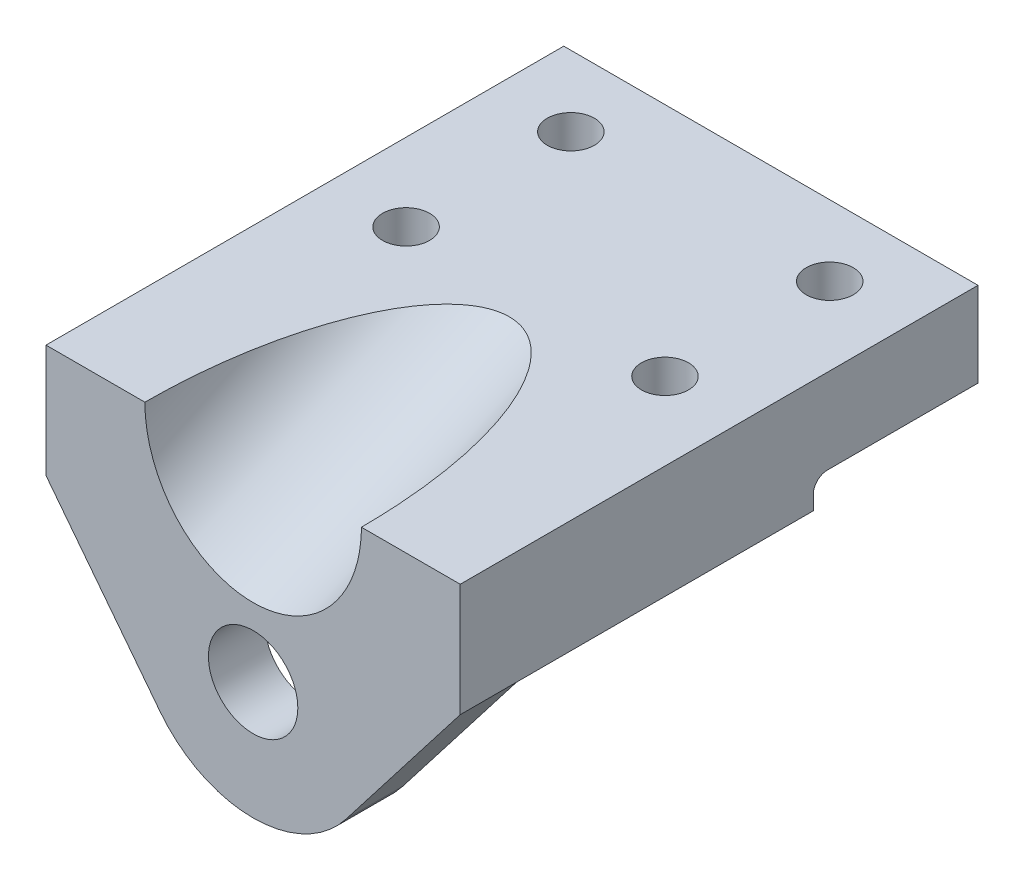
ISO-10303-21;
HEADER;
FILE_DESCRIPTION(('STEP AP214'),'2;1');
FILE_NAME('part.step','',(''),(''),'','','');
FILE_SCHEMA(('AUTOMOTIVE_DESIGN { 1 0 10303 214 1 1 1 1 }'));
ENDSEC;
DATA;
#1=APPLICATION_CONTEXT('core data for automotive mechanical design processes');
#2=APPLICATION_PROTOCOL_DEFINITION('international standard','automotive_design',2000,#1);
#3=PRODUCT_CONTEXT('',#1,'mechanical');
#4=PRODUCT('Part','Part','',(#3));
#5=PRODUCT_RELATED_PRODUCT_CATEGORY('part','',(#4));
#6=PRODUCT_DEFINITION_FORMATION('','',#4);
#7=PRODUCT_DEFINITION_CONTEXT('part definition',#1,'design');
#8=PRODUCT_DEFINITION('design','',#6,#7);
#9=PRODUCT_DEFINITION_SHAPE('','',#8);
#10=(LENGTH_UNIT() NAMED_UNIT(*) SI_UNIT(.MILLI.,.METRE.));
#11=(NAMED_UNIT(*) PLANE_ANGLE_UNIT() SI_UNIT($,.RADIAN.));
#12=(NAMED_UNIT(*) SI_UNIT($,.STERADIAN.) SOLID_ANGLE_UNIT());
#13=UNCERTAINTY_MEASURE_WITH_UNIT(LENGTH_MEASURE(1.E-05),#10,'distance_accuracy_value','');
#14=(GEOMETRIC_REPRESENTATION_CONTEXT(3) GLOBAL_UNCERTAINTY_ASSIGNED_CONTEXT((#13)) GLOBAL_UNIT_ASSIGNED_CONTEXT((#10,
#11,#12)) REPRESENTATION_CONTEXT('',''));
#15=CARTESIAN_POINT('',(0.,0.,0.));
#16=DIRECTION('',(0.,0.,1.));
#17=DIRECTION('',(1.,0.,0.));
#18=AXIS2_PLACEMENT_3D('',#15,#16,#17);
#19=CARTESIAN_POINT('',(-39.1308775839132,-30.2902442084566,-110.));
#20=DIRECTION('',(-0.790768984129773,-0.612114706356878,0.));
#21=DIRECTION('',(0.612114706356878,-0.790768984129773,0.));
#22=AXIS2_PLACEMENT_3D('',#19,#20,#21);
#23=PLANE('',#22);
#24=DIRECTION('',(-0.612114706356878,0.790768984129773,0.));
#25=VECTOR('',#24,1.);
#26=CARTESIAN_POINT('',(-39.1308775839132,-30.2902442084566,-12.));
#27=LINE('',#26,#25);
#28=CARTESIAN_POINT('',(-19.7692246032443,-55.3028676589219,-12.));
#29=VERTEX_POINT('',#28);
#30=CARTESIAN_POINT('',(-44.,-24.,-12.));
#31=VERTEX_POINT('',#30);
#32=EDGE_CURVE('E217',#29,#31,#27,.T.);
#33=ORIENTED_EDGE('',*,*,#32,.F.);
#34=DIRECTION('',(0.,0.,1.));
#35=VECTOR('',#34,1.);
#36=CARTESIAN_POINT('',(-19.7692246032443,-55.3028676589219,-110.));
#37=LINE('',#36,#35);
#38=CARTESIAN_POINT('',(-19.7692246032443,-55.3028676589219,0.));
#39=VERTEX_POINT('',#38);
#40=EDGE_CURVE('E163',#29,#39,#37,.T.);
#41=ORIENTED_EDGE('',*,*,#40,.T.);
#42=DIRECTION('',(0.612114706356878,-0.790768984129773,0.));
#43=VECTOR('',#42,1.);
#44=CARTESIAN_POINT('',(-39.1308775839132,-30.2902442084566,0.));
#45=LINE('',#44,#43);
#46=CARTESIAN_POINT('',(-44.,-24.,0.));
#47=VERTEX_POINT('',#46);
#48=EDGE_CURVE('E228',#47,#39,#45,.T.);
#49=ORIENTED_EDGE('',*,*,#48,.F.);
#50=DIRECTION('',(0.,0.,1.));
#51=VECTOR('',#50,1.);
#52=CARTESIAN_POINT('',(-44.,-24.,-110.));
#53=LINE('',#52,#51);
#54=EDGE_CURVE('E152',#31,#47,#53,.T.);
#55=ORIENTED_EDGE('',*,*,#54,.F.);
#56=EDGE_LOOP('',(#33,#41,#49,#55));
#57=FACE_BOUND('',#56,.T.);
#58=ADVANCED_FACE('F41',(#57),#23,.T.);
#59=CARTESIAN_POINT('',(-44.,0.,-110.));
#60=DIRECTION('',(-1.,0.,0.));
#61=DIRECTION('',(0.,-1.,0.));
#62=AXIS2_PLACEMENT_3D('',#59,#60,#61);
#63=PLANE('',#62);
#64=DIRECTION('',(0.,1.,0.));
#65=VECTOR('',#64,1.);
#66=CARTESIAN_POINT('',(-44.,0.,-75.));
#67=LINE('',#66,#65);
#68=CARTESIAN_POINT('',(-44.,-24.,-75.));
#69=VERTEX_POINT('',#68);
#70=CARTESIAN_POINT('',(-44.,-21.,-75.));
#71=VERTEX_POINT('',#70);
#72=EDGE_CURVE('E221',#69,#71,#67,.T.);
#73=ORIENTED_EDGE('',*,*,#72,.F.);
#74=DIRECTION('',(0.,0.,-1.));
#75=VECTOR('',#74,1.);
#76=CARTESIAN_POINT('',(-44.,-24.,-110.));
#77=LINE('',#76,#75);
#78=EDGE_CURVE('E219',#31,#69,#77,.T.);
#79=ORIENTED_EDGE('',*,*,#78,.F.);
#80=ORIENTED_EDGE('',*,*,#54,.T.);
#81=DIRECTION('',(0.,-1.,0.));
#82=VECTOR('',#81,1.);
#83=CARTESIAN_POINT('',(-44.,0.,0.));
#84=LINE('',#83,#82);
#85=CARTESIAN_POINT('',(-44.,0.,0.));
#86=VERTEX_POINT('',#85);
#87=EDGE_CURVE('E141',#86,#47,#84,.T.);
#88=ORIENTED_EDGE('',*,*,#87,.F.);
#89=DIRECTION('',(0.,0.,1.));
#90=VECTOR('',#89,1.);
#91=CARTESIAN_POINT('',(-44.,0.,-110.));
#92=LINE('',#91,#90);
#93=CARTESIAN_POINT('',(-44.,0.,-110.));
#94=VERTEX_POINT('',#93);
#95=EDGE_CURVE('E156',#94,#86,#92,.T.);
#96=ORIENTED_EDGE('',*,*,#95,.F.);
#97=DIRECTION('',(0.,-1.,0.));
#98=VECTOR('',#97,1.);
#99=CARTESIAN_POINT('',(-44.,0.,-110.));
#100=LINE('',#99,#98);
#101=CARTESIAN_POINT('',(-44.,-18.,-110.));
#102=VERTEX_POINT('',#101);
#103=EDGE_CURVE('E167',#94,#102,#100,.T.);
#104=ORIENTED_EDGE('',*,*,#103,.T.);
#105=DIRECTION('',(0.,0.,-1.));
#106=VECTOR('',#105,1.);
#107=CARTESIAN_POINT('',(-44.,-18.,-110.));
#108=LINE('',#107,#106);
#109=CARTESIAN_POINT('',(-44.,-18.,-78.));
#110=VERTEX_POINT('',#109);
#111=EDGE_CURVE('E61',#110,#102,#108,.T.);
#112=ORIENTED_EDGE('',*,*,#111,.F.);
#113=CARTESIAN_POINT('',(-44.,-21.,-78.));
#114=DIRECTION('',(-1.,0.,0.));
#115=DIRECTION('',(0.,-1.,0.));
#116=AXIS2_PLACEMENT_3D('',#113,#114,#115);
#117=CIRCLE('',#116,3.);
#118=EDGE_CURVE('E225',#71,#110,#117,.T.);
#119=ORIENTED_EDGE('',*,*,#118,.F.);
#120=EDGE_LOOP('',(#73,#79,#80,#88,#96,#104,#112,#119));
#121=FACE_BOUND('',#120,.T.);
#122=ADVANCED_FACE('F259',(#121),#63,.T.);
#123=CARTESIAN_POINT('',(0.,0.,-110.));
#124=DIRECTION('',(0.,-1.,0.));
#125=DIRECTION('',(0.,0.,-1.));
#126=AXIS2_PLACEMENT_3D('',#123,#124,#125);
#127=PLANE('',#126);
#128=CARTESIAN_POINT('',(27.5,0.,-95.));
#129=DIRECTION('',(0.,-1.,0.));
#130=DIRECTION('',(0.,0.,-1.));
#131=AXIS2_PLACEMENT_3D('',#128,#129,#130);
#132=CIRCLE('',#131,5.);
#133=CARTESIAN_POINT('',(27.5,0.,-100.));
#134=VERTEX_POINT('',#133);
#135=EDGE_CURVE('E176',#134,#134,#132,.T.);
#136=ORIENTED_EDGE('',*,*,#135,.T.);
#137=EDGE_LOOP('',(#136));
#138=FACE_BOUND('',#137,.T.);
#139=CARTESIAN_POINT('',(27.5,0.,-60.));
#140=DIRECTION('',(0.,-1.,0.));
#141=DIRECTION('',(0.,0.,-1.));
#142=AXIS2_PLACEMENT_3D('',#139,#140,#141);
#143=CIRCLE('',#142,5.);
#144=CARTESIAN_POINT('',(27.5,0.,-65.));
#145=VERTEX_POINT('',#144);
#146=EDGE_CURVE('E132',#145,#145,#143,.T.);
#147=ORIENTED_EDGE('',*,*,#146,.T.);
#148=EDGE_LOOP('',(#147));
#149=FACE_BOUND('',#148,.T.);
#150=CARTESIAN_POINT('',(-27.5,0.,-60.));
#151=DIRECTION('',(0.,-1.,0.));
#152=DIRECTION('',(0.,0.,-1.));
#153=AXIS2_PLACEMENT_3D('',#150,#151,#152);
#154=CIRCLE('',#153,5.);
#155=CARTESIAN_POINT('',(-27.5,0.,-65.));
#156=VERTEX_POINT('',#155);
#157=EDGE_CURVE('E182',#156,#156,#154,.T.);
#158=ORIENTED_EDGE('',*,*,#157,.T.);
#159=EDGE_LOOP('',(#158));
#160=FACE_BOUND('',#159,.T.);
#161=CARTESIAN_POINT('',(-27.5,0.,-95.));
#162=DIRECTION('',(0.,-1.,0.));
#163=DIRECTION('',(0.,0.,-1.));
#164=AXIS2_PLACEMENT_3D('',#161,#162,#163);
#165=CIRCLE('',#164,5.);
#166=CARTESIAN_POINT('',(-27.5,0.,-100.));
#167=VERTEX_POINT('',#166);
#168=EDGE_CURVE('E174',#167,#167,#165,.T.);
#169=ORIENTED_EDGE('',*,*,#168,.T.);
#170=EDGE_LOOP('',(#169));
#171=FACE_BOUND('',#170,.T.);
#172=DIRECTION('',(1.,0.,0.));
#173=VECTOR('',#172,1.);
#174=CARTESIAN_POINT('',(0.,0.,0.));
#175=LINE('',#174,#173);
#176=CARTESIAN_POINT('',(-23.,0.,0.));
#177=VERTEX_POINT('',#176);
#178=EDGE_CURVE('E135',#86,#177,#175,.T.);
#179=ORIENTED_EDGE('',*,*,#178,.T.);
#180=CARTESIAN_POINT('',(0.,0.,0.));
#181=DIRECTION('',(0.,-1.,0.));
#182=DIRECTION('',(0.,0.,-1.));
#183=AXIS2_PLACEMENT_3D('',#180,#181,#182);
#184=ELLIPSE('',#183,54.4226364125082,23.);
#185=CARTESIAN_POINT('',(23.,0.,0.));
#186=VERTEX_POINT('',#185);
#187=EDGE_CURVE('E54',#177,#186,#184,.T.);
#188=ORIENTED_EDGE('',*,*,#187,.T.);
#189=CARTESIAN_POINT('',(44.,0.,0.));
#190=VERTEX_POINT('',#189);
#191=EDGE_CURVE('E128',#186,#190,#175,.T.);
#192=ORIENTED_EDGE('',*,*,#191,.T.);
#193=DIRECTION('',(0.,0.,1.));
#194=VECTOR('',#193,1.);
#195=CARTESIAN_POINT('',(44.,0.,-110.));
#196=LINE('',#195,#194);
#197=CARTESIAN_POINT('',(44.,0.,-110.));
#198=VERTEX_POINT('',#197);
#199=EDGE_CURVE('E158',#198,#190,#196,.T.);
#200=ORIENTED_EDGE('',*,*,#199,.F.);
#201=DIRECTION('',(1.,0.,0.));
#202=VECTOR('',#201,1.);
#203=CARTESIAN_POINT('',(0.,0.,-110.));
#204=LINE('',#203,#202);
#205=EDGE_CURVE('E227',#94,#198,#204,.T.);
#206=ORIENTED_EDGE('',*,*,#205,.F.);
#207=ORIENTED_EDGE('',*,*,#95,.T.);
#208=EDGE_LOOP('',(#179,#188,#192,#200,#206,#207));
#209=FACE_BOUND('',#208,.T.);
#210=ADVANCED_FACE('F126',(#138,#149,#160,#171,#209),#127,.F.);
#211=CARTESIAN_POINT('',(44.,0.,-110.));
#212=DIRECTION('',(-1.,0.,0.));
#213=DIRECTION('',(0.,-1.,0.));
#214=AXIS2_PLACEMENT_3D('',#211,#212,#213);
#215=PLANE('',#214);
#216=DIRECTION('',(0.,0.,1.));
#217=VECTOR('',#216,1.);
#218=CARTESIAN_POINT('',(44.,-24.,-12.));
#219=LINE('',#218,#217);
#220=CARTESIAN_POINT('',(44.,-24.,-75.));
#221=VERTEX_POINT('',#220);
#222=CARTESIAN_POINT('',(44.,-24.,-12.));
#223=VERTEX_POINT('',#222);
#224=EDGE_CURVE('E205',#221,#223,#219,.T.);
#225=ORIENTED_EDGE('',*,*,#224,.F.);
#226=DIRECTION('',(0.,-1.,0.));
#227=VECTOR('',#226,1.);
#228=CARTESIAN_POINT('',(44.,-24.,-75.));
#229=LINE('',#228,#227);
#230=CARTESIAN_POINT('',(44.,-21.,-75.));
#231=VERTEX_POINT('',#230);
#232=EDGE_CURVE('E200',#231,#221,#229,.T.);
#233=ORIENTED_EDGE('',*,*,#232,.F.);
#234=CARTESIAN_POINT('',(44.,-21.,-78.));
#235=DIRECTION('',(1.,0.,0.));
#236=DIRECTION('',(0.,-1.,0.));
#237=AXIS2_PLACEMENT_3D('',#234,#235,#236);
#238=CIRCLE('',#237,3.);
#239=CARTESIAN_POINT('',(44.,-18.,-78.));
#240=VERTEX_POINT('',#239);
#241=EDGE_CURVE('E198',#240,#231,#238,.T.);
#242=ORIENTED_EDGE('',*,*,#241,.F.);
#243=DIRECTION('',(0.,0.,1.));
#244=VECTOR('',#243,1.);
#245=CARTESIAN_POINT('',(44.,-18.,-78.));
#246=LINE('',#245,#244);
#247=CARTESIAN_POINT('',(44.,-18.,-110.));
#248=VERTEX_POINT('',#247);
#249=EDGE_CURVE('E131',#248,#240,#246,.T.);
#250=ORIENTED_EDGE('',*,*,#249,.F.);
#251=DIRECTION('',(0.,-1.,0.));
#252=VECTOR('',#251,1.);
#253=CARTESIAN_POINT('',(44.,0.,-110.));
#254=LINE('',#253,#252);
#255=EDGE_CURVE('E153',#198,#248,#254,.T.);
#256=ORIENTED_EDGE('',*,*,#255,.F.);
#257=ORIENTED_EDGE('',*,*,#199,.T.);
#258=DIRECTION('',(0.,-1.,0.));
#259=VECTOR('',#258,1.);
#260=CARTESIAN_POINT('',(44.,0.,0.));
#261=LINE('',#260,#259);
#262=CARTESIAN_POINT('',(44.,-24.,0.));
#263=VERTEX_POINT('',#262);
#264=EDGE_CURVE('E143',#190,#263,#261,.T.);
#265=ORIENTED_EDGE('',*,*,#264,.T.);
#266=DIRECTION('',(0.,0.,1.));
#267=VECTOR('',#266,1.);
#268=CARTESIAN_POINT('',(44.,-24.,-110.));
#269=LINE('',#268,#267);
#270=EDGE_CURVE('E159',#223,#263,#269,.T.);
#271=ORIENTED_EDGE('',*,*,#270,.F.);
#272=EDGE_LOOP('',(#225,#233,#242,#250,#256,#257,#265,#271));
#273=FACE_BOUND('',#272,.T.);
#274=ADVANCED_FACE('F271',(#273),#215,.F.);
#275=CARTESIAN_POINT('',(39.1308775839132,-30.2902442084566,-110.));
#276=DIRECTION('',(-0.790768984129773,0.612114706356877,0.));
#277=DIRECTION('',(-0.612114706356877,-0.790768984129773,0.));
#278=AXIS2_PLACEMENT_3D('',#275,#276,#277);
#279=PLANE('',#278);
#280=DIRECTION('',(0.,0.,1.));
#281=VECTOR('',#280,1.);
#282=CARTESIAN_POINT('',(19.7692246032443,-55.3028676589219,-110.));
#283=LINE('',#282,#281);
#284=CARTESIAN_POINT('',(19.7692246032443,-55.3028676589219,-12.));
#285=VERTEX_POINT('',#284);
#286=CARTESIAN_POINT('',(19.7692246032443,-55.3028676589219,0.));
#287=VERTEX_POINT('',#286);
#288=EDGE_CURVE('E165',#285,#287,#283,.T.);
#289=ORIENTED_EDGE('',*,*,#288,.F.);
#290=DIRECTION('',(0.612114706356877,0.790768984129773,0.));
#291=VECTOR('',#290,1.);
#292=CARTESIAN_POINT('',(39.1308775839132,-30.2902442084566,-12.));
#293=LINE('',#292,#291);
#294=EDGE_CURVE('E214',#285,#223,#293,.T.);
#295=ORIENTED_EDGE('',*,*,#294,.T.);
#296=ORIENTED_EDGE('',*,*,#270,.T.);
#297=DIRECTION('',(-0.612114706356877,-0.790768984129774,0.));
#298=VECTOR('',#297,1.);
#299=CARTESIAN_POINT('',(39.1308775839132,-30.2902442084566,0.));
#300=LINE('',#299,#298);
#301=EDGE_CURVE('E145',#263,#287,#300,.T.);
#302=ORIENTED_EDGE('',*,*,#301,.T.);
#303=EDGE_LOOP('',(#289,#295,#296,#302));
#304=FACE_BOUND('',#303,.T.);
#305=ADVANCED_FACE('F238',(#304),#279,.F.);
#306=CARTESIAN_POINT('',(0.,-40.,-110.));
#307=DIRECTION('',(0.,0.,1.));
#308=DIRECTION('',(1.,0.,0.));
#309=AXIS2_PLACEMENT_3D('',#306,#307,#308);
#310=CYLINDRICAL_SURFACE('',#309,25.);
#311=CARTESIAN_POINT('',(0.,-40.,-12.));
#312=DIRECTION('',(0.,0.,1.));
#313=DIRECTION('',(1.,0.,0.));
#314=AXIS2_PLACEMENT_3D('',#311,#312,#313);
#315=CIRCLE('',#314,25.);
#316=EDGE_CURVE('E168',#285,#29,#315,.F.);
#317=ORIENTED_EDGE('',*,*,#316,.F.);
#318=ORIENTED_EDGE('',*,*,#288,.T.);
#319=CARTESIAN_POINT('',(0.,-40.,0.));
#320=DIRECTION('',(0.,0.,1.));
#321=DIRECTION('',(1.,0.,0.));
#322=AXIS2_PLACEMENT_3D('',#319,#320,#321);
#323=CIRCLE('',#322,25.);
#324=EDGE_CURVE('E232',#39,#287,#323,.T.);
#325=ORIENTED_EDGE('',*,*,#324,.F.);
#326=ORIENTED_EDGE('',*,*,#40,.F.);
#327=EDGE_LOOP('',(#317,#318,#325,#326));
#328=FACE_BOUND('',#327,.T.);
#329=ADVANCED_FACE('F250',(#328),#310,.T.);
#330=CARTESIAN_POINT('',(0.,-40.,-110.));
#331=DIRECTION('',(0.,0.,1.));
#332=DIRECTION('',(1.,0.,0.));
#333=AXIS2_PLACEMENT_3D('',#330,#331,#332);
#334=CYLINDRICAL_SURFACE('',#333,9.5);
#335=CARTESIAN_POINT('',(0.,-40.,-12.));
#336=DIRECTION('',(0.,0.,1.));
#337=DIRECTION('',(1.,0.,0.));
#338=AXIS2_PLACEMENT_3D('',#335,#336,#337);
#339=CIRCLE('',#338,9.5);
#340=CARTESIAN_POINT('',(9.50000000000001,-40.,-12.));
#341=VERTEX_POINT('',#340);
#342=EDGE_CURVE('E169',#341,#341,#339,.F.);
#343=ORIENTED_EDGE('',*,*,#342,.T.);
#344=EDGE_LOOP('',(#343));
#345=FACE_BOUND('',#344,.T.);
#346=CARTESIAN_POINT('',(0.,-40.,0.));
#347=DIRECTION('',(0.,0.,1.));
#348=DIRECTION('',(1.,0.,0.));
#349=AXIS2_PLACEMENT_3D('',#346,#347,#348);
#350=CIRCLE('',#349,9.5);
#351=CARTESIAN_POINT('',(9.50000000000001,-40.,0.));
#352=VERTEX_POINT('',#351);
#353=EDGE_CURVE('E147',#352,#352,#350,.T.);
#354=ORIENTED_EDGE('',*,*,#353,.T.);
#355=EDGE_LOOP('',(#354));
#356=FACE_BOUND('',#355,.T.);
#357=ADVANCED_FACE('F308',(#345,#356),#334,.F.);
#358=CARTESIAN_POINT('',(0.,0.,-110.));
#359=DIRECTION('',(0.,0.,1.));
#360=DIRECTION('',(1.,0.,0.));
#361=AXIS2_PLACEMENT_3D('',#358,#359,#360);
#362=PLANE('',#361);
#363=ORIENTED_EDGE('',*,*,#255,.T.);
#364=DIRECTION('',(-1.,0.,0.));
#365=VECTOR('',#364,1.);
#366=CARTESIAN_POINT('',(0.,-18.,-110.));
#367=LINE('',#366,#365);
#368=EDGE_CURVE('E47',#248,#102,#367,.T.);
#369=ORIENTED_EDGE('',*,*,#368,.T.);
#370=ORIENTED_EDGE('',*,*,#103,.F.);
#371=ORIENTED_EDGE('',*,*,#205,.T.);
#372=EDGE_LOOP('',(#363,#369,#370,#371));
#373=FACE_BOUND('',#372,.T.);
#374=ADVANCED_FACE('F280',(#373),#362,.F.);
#375=CARTESIAN_POINT('',(0.,0.,0.));
#376=DIRECTION('',(0.,0.,1.));
#377=DIRECTION('',(1.,0.,0.));
#378=AXIS2_PLACEMENT_3D('',#375,#376,#377);
#379=PLANE('',#378);
#380=CARTESIAN_POINT('',(0.,0.,0.));
#381=DIRECTION('',(0.,0.,1.));
#382=DIRECTION('',(0.,1.,0.));
#383=AXIS2_PLACEMENT_3D('',#380,#381,#382);
#384=ELLIPSE('',#383,25.3776921361372,23.);
#385=EDGE_CURVE('E11',#177,#186,#384,.T.);
#386=ORIENTED_EDGE('',*,*,#385,.F.);
#387=ORIENTED_EDGE('',*,*,#178,.F.);
#388=ORIENTED_EDGE('',*,*,#87,.T.);
#389=ORIENTED_EDGE('',*,*,#48,.T.);
#390=ORIENTED_EDGE('',*,*,#324,.T.);
#391=ORIENTED_EDGE('',*,*,#301,.F.);
#392=ORIENTED_EDGE('',*,*,#264,.F.);
#393=ORIENTED_EDGE('',*,*,#191,.F.);
#394=EDGE_LOOP('',(#386,#387,#388,#389,#390,#391,#392,#393));
#395=FACE_BOUND('',#394,.T.);
#396=ORIENTED_EDGE('',*,*,#353,.F.);
#397=EDGE_LOOP('',(#396));
#398=FACE_BOUND('',#397,.T.);
#399=ADVANCED_FACE('F140',(#395,#398),#379,.T.);
#400=CARTESIAN_POINT('',(-66.,-76.3599593142704,-12.));
#401=DIRECTION('',(0.,0.,1.));
#402=DIRECTION('',(1.,0.,0.));
#403=AXIS2_PLACEMENT_3D('',#400,#401,#402);
#404=PLANE('',#403);
#405=ORIENTED_EDGE('',*,*,#32,.T.);
#406=DIRECTION('',(1.,0.,0.));
#407=VECTOR('',#406,1.);
#408=CARTESIAN_POINT('',(-66.,-24.,-12.));
#409=LINE('',#408,#407);
#410=EDGE_CURVE('E206',#31,#223,#409,.T.);
#411=ORIENTED_EDGE('',*,*,#410,.T.);
#412=ORIENTED_EDGE('',*,*,#294,.F.);
#413=ORIENTED_EDGE('',*,*,#316,.T.);
#414=EDGE_LOOP('',(#405,#411,#412,#413));
#415=FACE_BOUND('',#414,.T.);
#416=ORIENTED_EDGE('',*,*,#342,.F.);
#417=EDGE_LOOP('',(#416));
#418=FACE_BOUND('',#417,.T.);
#419=ADVANCED_FACE('F247',(#415,#418),#404,.F.);
#420=CARTESIAN_POINT('',(-66.,-24.,-12.));
#421=DIRECTION('',(0.,1.,0.));
#422=DIRECTION('',(-1.,0.,0.));
#423=AXIS2_PLACEMENT_3D('',#420,#421,#422);
#424=PLANE('',#423);
#425=CARTESIAN_POINT('',(27.5,-24.,-60.));
#426=DIRECTION('',(0.,1.,0.));
#427=DIRECTION('',(-1.,0.,0.));
#428=AXIS2_PLACEMENT_3D('',#425,#426,#427);
#429=CIRCLE('',#428,5.);
#430=CARTESIAN_POINT('',(22.5,-24.,-60.));
#431=VERTEX_POINT('',#430);
#432=EDGE_CURVE('E42',#431,#431,#429,.T.);
#433=ORIENTED_EDGE('',*,*,#432,.T.);
#434=EDGE_LOOP('',(#433));
#435=FACE_BOUND('',#434,.T.);
#436=CARTESIAN_POINT('',(-27.5,-24.,-60.));
#437=DIRECTION('',(0.,1.,0.));
#438=DIRECTION('',(-1.,0.,0.));
#439=AXIS2_PLACEMENT_3D('',#436,#437,#438);
#440=CIRCLE('',#439,5.);
#441=CARTESIAN_POINT('',(-32.5,-24.,-60.));
#442=VERTEX_POINT('',#441);
#443=EDGE_CURVE('E179',#442,#442,#440,.T.);
#444=ORIENTED_EDGE('',*,*,#443,.T.);
#445=EDGE_LOOP('',(#444));
#446=FACE_BOUND('',#445,.T.);
#447=ORIENTED_EDGE('',*,*,#78,.T.);
#448=DIRECTION('',(1.,0.,0.));
#449=VECTOR('',#448,1.);
#450=CARTESIAN_POINT('',(-66.,-24.,-75.));
#451=LINE('',#450,#449);
#452=EDGE_CURVE('E208',#69,#221,#451,.T.);
#453=ORIENTED_EDGE('',*,*,#452,.T.);
#454=ORIENTED_EDGE('',*,*,#224,.T.);
#455=ORIENTED_EDGE('',*,*,#410,.F.);
#456=EDGE_LOOP('',(#447,#453,#454,#455));
#457=FACE_BOUND('',#456,.T.);
#458=ADVANCED_FACE('F263',(#435,#446,#457),#424,.F.);
#459=CARTESIAN_POINT('',(-66.,-24.,-75.));
#460=DIRECTION('',(0.,0.,1.));
#461=DIRECTION('',(1.,0.,0.));
#462=AXIS2_PLACEMENT_3D('',#459,#460,#461);
#463=PLANE('',#462);
#464=ORIENTED_EDGE('',*,*,#72,.T.);
#465=DIRECTION('',(1.,0.,0.));
#466=VECTOR('',#465,1.);
#467=CARTESIAN_POINT('',(-66.,-21.0000000000001,-75.));
#468=LINE('',#467,#466);
#469=EDGE_CURVE('E209',#71,#231,#468,.T.);
#470=ORIENTED_EDGE('',*,*,#469,.T.);
#471=ORIENTED_EDGE('',*,*,#232,.T.);
#472=ORIENTED_EDGE('',*,*,#452,.F.);
#473=EDGE_LOOP('',(#464,#470,#471,#472));
#474=FACE_BOUND('',#473,.T.);
#475=ADVANCED_FACE('F264',(#474),#463,.F.);
#476=CARTESIAN_POINT('',(-66.,-21.,-78.));
#477=DIRECTION('',(1.,0.,0.));
#478=DIRECTION('',(0.,1.,0.));
#479=AXIS2_PLACEMENT_3D('',#476,#477,#478);
#480=CYLINDRICAL_SURFACE('',#479,3.);
#481=ORIENTED_EDGE('',*,*,#118,.T.);
#482=DIRECTION('',(1.,0.,0.));
#483=VECTOR('',#482,1.);
#484=CARTESIAN_POINT('',(-66.,-18.,-78.));
#485=LINE('',#484,#483);
#486=EDGE_CURVE('E202',#110,#240,#485,.T.);
#487=ORIENTED_EDGE('',*,*,#486,.T.);
#488=ORIENTED_EDGE('',*,*,#241,.T.);
#489=ORIENTED_EDGE('',*,*,#469,.F.);
#490=EDGE_LOOP('',(#481,#487,#488,#489));
#491=FACE_BOUND('',#490,.T.);
#492=ADVANCED_FACE('F276',(#491),#480,.F.);
#493=CARTESIAN_POINT('',(-66.,-18.,-78.));
#494=DIRECTION('',(0.,1.,0.));
#495=DIRECTION('',(-1.,0.,0.));
#496=AXIS2_PLACEMENT_3D('',#493,#494,#495);
#497=PLANE('',#496);
#498=CARTESIAN_POINT('',(27.5,-18.,-95.));
#499=DIRECTION('',(0.,1.,0.));
#500=DIRECTION('',(-1.,0.,0.));
#501=AXIS2_PLACEMENT_3D('',#498,#499,#500);
#502=CIRCLE('',#501,5.);
#503=CARTESIAN_POINT('',(22.5,-18.,-95.));
#504=VERTEX_POINT('',#503);
#505=EDGE_CURVE('E178',#504,#504,#502,.T.);
#506=ORIENTED_EDGE('',*,*,#505,.T.);
#507=EDGE_LOOP('',(#506));
#508=FACE_BOUND('',#507,.T.);
#509=CARTESIAN_POINT('',(-27.5,-18.,-95.));
#510=DIRECTION('',(0.,1.,0.));
#511=DIRECTION('',(-1.,0.,0.));
#512=AXIS2_PLACEMENT_3D('',#509,#510,#511);
#513=CIRCLE('',#512,5.);
#514=CARTESIAN_POINT('',(-32.5,-18.,-95.));
#515=VERTEX_POINT('',#514);
#516=EDGE_CURVE('E175',#515,#515,#513,.T.);
#517=ORIENTED_EDGE('',*,*,#516,.T.);
#518=EDGE_LOOP('',(#517));
#519=FACE_BOUND('',#518,.T.);
#520=ORIENTED_EDGE('',*,*,#111,.T.);
#521=ORIENTED_EDGE('',*,*,#368,.F.);
#522=ORIENTED_EDGE('',*,*,#249,.T.);
#523=ORIENTED_EDGE('',*,*,#486,.F.);
#524=EDGE_LOOP('',(#520,#521,#522,#523));
#525=FACE_BOUND('',#524,.T.);
#526=ADVANCED_FACE('F278',(#508,#519,#525),#497,.F.);
#527=CARTESIAN_POINT('',(0.,-23.2440043957382,49.8469282870159));
#528=DIRECTION('',(0.,0.422618261740694,-0.906307787036653));
#529=DIRECTION('',(0.,0.906307787036653,0.422618261740694));
#530=AXIS2_PLACEMENT_3D('',#527,#528,#529);
#531=CYLINDRICAL_SURFACE('',#530,23.);
#532=ORIENTED_EDGE('',*,*,#385,.T.);
#533=ORIENTED_EDGE('',*,*,#187,.F.);
#534=EDGE_LOOP('',(#532,#533));
#535=FACE_BOUND('',#534,.T.);
#536=ADVANCED_FACE('F125',(#535),#531,.F.);
#537=CARTESIAN_POINT('',(-27.5,-55.,-95.));
#538=DIRECTION('',(0.,1.,0.));
#539=DIRECTION('',(0.,0.,1.));
#540=AXIS2_PLACEMENT_3D('',#537,#538,#539);
#541=CYLINDRICAL_SURFACE('',#540,5.);
#542=ORIENTED_EDGE('',*,*,#516,.F.);
#543=EDGE_LOOP('',(#542));
#544=FACE_BOUND('',#543,.T.);
#545=ORIENTED_EDGE('',*,*,#168,.F.);
#546=EDGE_LOOP('',(#545));
#547=FACE_BOUND('',#546,.T.);
#548=ADVANCED_FACE('F289',(#544,#547),#541,.F.);
#549=CARTESIAN_POINT('',(27.5,-55.,-95.));
#550=DIRECTION('',(0.,1.,0.));
#551=DIRECTION('',(0.,0.,1.));
#552=AXIS2_PLACEMENT_3D('',#549,#550,#551);
#553=CYLINDRICAL_SURFACE('',#552,5.);
#554=ORIENTED_EDGE('',*,*,#505,.F.);
#555=EDGE_LOOP('',(#554));
#556=FACE_BOUND('',#555,.T.);
#557=ORIENTED_EDGE('',*,*,#135,.F.);
#558=EDGE_LOOP('',(#557));
#559=FACE_BOUND('',#558,.T.);
#560=ADVANCED_FACE('F363',(#556,#559),#553,.F.);
#561=CARTESIAN_POINT('',(-27.5,-55.,-60.));
#562=DIRECTION('',(0.,1.,0.));
#563=DIRECTION('',(0.,0.,1.));
#564=AXIS2_PLACEMENT_3D('',#561,#562,#563);
#565=CYLINDRICAL_SURFACE('',#564,5.);
#566=ORIENTED_EDGE('',*,*,#443,.F.);
#567=EDGE_LOOP('',(#566));
#568=FACE_BOUND('',#567,.T.);
#569=ORIENTED_EDGE('',*,*,#157,.F.);
#570=EDGE_LOOP('',(#569));
#571=FACE_BOUND('',#570,.T.);
#572=ADVANCED_FACE('F367',(#568,#571),#565,.F.);
#573=CARTESIAN_POINT('',(27.5,-55.,-60.));
#574=DIRECTION('',(0.,1.,0.));
#575=DIRECTION('',(0.,0.,1.));
#576=AXIS2_PLACEMENT_3D('',#573,#574,#575);
#577=CYLINDRICAL_SURFACE('',#576,5.);
#578=ORIENTED_EDGE('',*,*,#432,.F.);
#579=EDGE_LOOP('',(#578));
#580=FACE_BOUND('',#579,.T.);
#581=ORIENTED_EDGE('',*,*,#146,.F.);
#582=EDGE_LOOP('',(#581));
#583=FACE_BOUND('',#582,.T.);
#584=ADVANCED_FACE('F379',(#580,#583),#577,.F.);
#585=CLOSED_SHELL('',(#58,#122,#210,#274,#305,#329,#357,#374,#399,#419,#458,#475,#492,#526,#536,
#548,#560,#572,#584));
#586=MANIFOLD_SOLID_BREP('B2',#585);
#587=ADVANCED_BREP_SHAPE_REPRESENTATION('',(#18,#586),#14);
#588=SHAPE_DEFINITION_REPRESENTATION(#9,#587);
ENDSEC;
END-ISO-10303-21;
